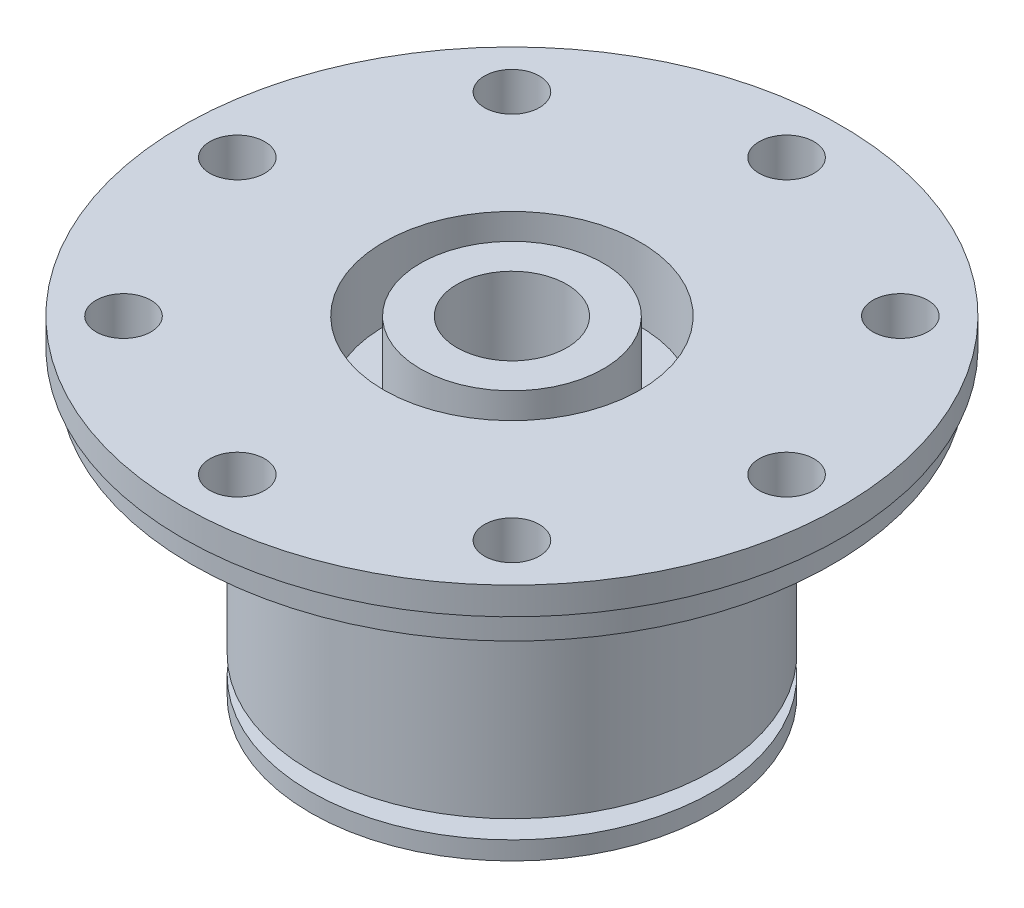
ISO-10303-21;
HEADER;
FILE_DESCRIPTION(('STEP AP214'),'2;1');
FILE_NAME('part.step','',(''),(''),'','','');
FILE_SCHEMA(('AUTOMOTIVE_DESIGN { 1 0 10303 214 1 1 1 1 }'));
ENDSEC;
DATA;
#1=APPLICATION_CONTEXT('core data for automotive mechanical design processes');
#2=APPLICATION_PROTOCOL_DEFINITION('international standard','automotive_design',2000,#1);
#3=PRODUCT_CONTEXT('',#1,'mechanical');
#4=PRODUCT('Part','Part','',(#3));
#5=PRODUCT_RELATED_PRODUCT_CATEGORY('part','',(#4));
#6=PRODUCT_DEFINITION_FORMATION('','',#4);
#7=PRODUCT_DEFINITION_CONTEXT('part definition',#1,'design');
#8=PRODUCT_DEFINITION('design','',#6,#7);
#9=PRODUCT_DEFINITION_SHAPE('','',#8);
#10=(LENGTH_UNIT() NAMED_UNIT(*) SI_UNIT(.MILLI.,.METRE.));
#11=(NAMED_UNIT(*) PLANE_ANGLE_UNIT() SI_UNIT($,.RADIAN.));
#12=(NAMED_UNIT(*) SI_UNIT($,.STERADIAN.) SOLID_ANGLE_UNIT());
#13=UNCERTAINTY_MEASURE_WITH_UNIT(LENGTH_MEASURE(1.E-05),#10,'distance_accuracy_value','');
#14=(GEOMETRIC_REPRESENTATION_CONTEXT(3) GLOBAL_UNCERTAINTY_ASSIGNED_CONTEXT((#13)) GLOBAL_UNIT_ASSIGNED_CONTEXT((#10,
#11,#12)) REPRESENTATION_CONTEXT('',''));
#15=CARTESIAN_POINT('',(0.,0.,0.));
#16=DIRECTION('',(0.,0.,1.));
#17=DIRECTION('',(1.,0.,0.));
#18=AXIS2_PLACEMENT_3D('',#15,#16,#17);
#19=CARTESIAN_POINT('',(-3.,7.42,-3.));
#20=DIRECTION('',(0.,1.,0.));
#21=DIRECTION('',(0.,0.,1.));
#22=AXIS2_PLACEMENT_3D('',#19,#20,#21);
#23=PLANE('',#22);
#24=DIRECTION('',(-1.,0.,0.));
#25=VECTOR('',#24,1.);
#26=CARTESIAN_POINT('',(-3.,7.42,3.));
#27=LINE('',#26,#25);
#28=CARTESIAN_POINT('',(3.,7.42,3.));
#29=VERTEX_POINT('',#28);
#30=CARTESIAN_POINT('',(0.,7.42,3.));
#31=VERTEX_POINT('',#30);
#32=EDGE_CURVE('E106',#29,#31,#27,.T.);
#33=ORIENTED_EDGE('',*,*,#32,.T.);
#34=CARTESIAN_POINT('',(0.,7.42,0.));
#35=DIRECTION('',(0.,1.,0.));
#36=DIRECTION('',(0.,0.,1.));
#37=AXIS2_PLACEMENT_3D('',#34,#35,#36);
#38=CIRCLE('',#37,3.);
#39=CARTESIAN_POINT('',(3.,7.42,0.));
#40=VERTEX_POINT('',#39);
#41=EDGE_CURVE('E53',#31,#40,#38,.T.);
#42=ORIENTED_EDGE('',*,*,#41,.T.);
#43=DIRECTION('',(0.,0.,1.));
#44=VECTOR('',#43,1.);
#45=CARTESIAN_POINT('',(3.,7.42,-3.));
#46=LINE('',#45,#44);
#47=EDGE_CURVE('E104',#40,#29,#46,.T.);
#48=ORIENTED_EDGE('',*,*,#47,.T.);
#49=EDGE_LOOP('',(#33,#42,#48));
#50=FACE_BOUND('',#49,.T.);
#51=ADVANCED_FACE('F39',(#50),#23,.F.);
#52=CARTESIAN_POINT('',(3.,7.42,-3.));
#53=VERTEX_POINT('',#52);
#54=EDGE_CURVE('E112',#53,#40,#46,.T.);
#55=ORIENTED_EDGE('',*,*,#54,.T.);
#56=CARTESIAN_POINT('',(0.,7.42,-3.));
#57=VERTEX_POINT('',#56);
#58=EDGE_CURVE('E95',#40,#57,#38,.T.);
#59=ORIENTED_EDGE('',*,*,#58,.T.);
#60=DIRECTION('',(-1.,0.,0.));
#61=VECTOR('',#60,1.);
#62=CARTESIAN_POINT('',(-3.,7.42,-3.));
#63=LINE('',#62,#61);
#64=EDGE_CURVE('E117',#53,#57,#63,.T.);
#65=ORIENTED_EDGE('',*,*,#64,.F.);
#66=EDGE_LOOP('',(#55,#59,#65));
#67=FACE_BOUND('',#66,.T.);
#68=ADVANCED_FACE('F111',(#67),#23,.F.);
#69=CARTESIAN_POINT('',(-3.,7.42,-3.));
#70=VERTEX_POINT('',#69);
#71=EDGE_CURVE('E208',#57,#70,#63,.T.);
#72=ORIENTED_EDGE('',*,*,#71,.F.);
#73=CARTESIAN_POINT('',(-3.,7.42,0.));
#74=VERTEX_POINT('',#73);
#75=EDGE_CURVE('E96',#57,#74,#38,.T.);
#76=ORIENTED_EDGE('',*,*,#75,.T.);
#77=DIRECTION('',(0.,0.,1.));
#78=VECTOR('',#77,1.);
#79=CARTESIAN_POINT('',(-3.,7.42,-3.));
#80=LINE('',#79,#78);
#81=EDGE_CURVE('E116',#70,#74,#80,.T.);
#82=ORIENTED_EDGE('',*,*,#81,.F.);
#83=EDGE_LOOP('',(#72,#76,#82));
#84=FACE_BOUND('',#83,.T.);
#85=ADVANCED_FACE('F184',(#84),#23,.F.);
#86=CARTESIAN_POINT('',(0.,1.,0.));
#87=DIRECTION('',(0.,-1.,0.));
#88=DIRECTION('',(0.,0.,-1.));
#89=AXIS2_PLACEMENT_3D('',#86,#87,#88);
#90=CYLINDRICAL_SURFACE('',#89,11.);
#91=CARTESIAN_POINT('',(0.,1.,0.));
#92=DIRECTION('',(0.,1.,0.));
#93=DIRECTION('',(0.,0.,1.));
#94=AXIS2_PLACEMENT_3D('',#91,#92,#93);
#95=CIRCLE('',#94,11.);
#96=CARTESIAN_POINT('',(0.,1.,11.));
#97=VERTEX_POINT('',#96);
#98=EDGE_CURVE('E152',#97,#97,#95,.T.);
#99=ORIENTED_EDGE('',*,*,#98,.F.);
#100=EDGE_LOOP('',(#99));
#101=FACE_BOUND('',#100,.T.);
#102=CARTESIAN_POINT('',(0.,0.,0.));
#103=DIRECTION('',(0.,1.,0.));
#104=DIRECTION('',(0.,0.,1.));
#105=AXIS2_PLACEMENT_3D('',#102,#103,#104);
#106=CIRCLE('',#105,11.);
#107=CARTESIAN_POINT('',(0.,0.,11.));
#108=VERTEX_POINT('',#107);
#109=EDGE_CURVE('E151',#108,#108,#106,.T.);
#110=ORIENTED_EDGE('',*,*,#109,.T.);
#111=EDGE_LOOP('',(#110));
#112=FACE_BOUND('',#111,.T.);
#113=ADVANCED_FACE('F41',(#101,#112),#90,.T.);
#114=CARTESIAN_POINT('',(0.,1.,0.));
#115=DIRECTION('',(0.,1.,0.));
#116=DIRECTION('',(0.,0.,1.));
#117=AXIS2_PLACEMENT_3D('',#114,#115,#116);
#118=PLANE('',#117);
#119=CARTESIAN_POINT('',(0.,1.,0.));
#120=DIRECTION('',(0.,1.,0.));
#121=DIRECTION('',(0.,0.,1.));
#122=AXIS2_PLACEMENT_3D('',#119,#120,#121);
#123=CIRCLE('',#122,9.5);
#124=CARTESIAN_POINT('',(0.,1.,9.5));
#125=VERTEX_POINT('',#124);
#126=EDGE_CURVE('E50',#125,#125,#123,.T.);
#127=ORIENTED_EDGE('',*,*,#126,.F.);
#128=EDGE_LOOP('',(#127));
#129=FACE_BOUND('',#128,.T.);
#130=ORIENTED_EDGE('',*,*,#98,.T.);
#131=EDGE_LOOP('',(#130));
#132=FACE_BOUND('',#131,.T.);
#133=ADVANCED_FACE('F162',(#129,#132),#118,.T.);
#134=CARTESIAN_POINT('',(0.,0.,0.));
#135=DIRECTION('',(0.,1.,0.));
#136=DIRECTION('',(0.,0.,1.));
#137=AXIS2_PLACEMENT_3D('',#134,#135,#136);
#138=PLANE('',#137);
#139=DIRECTION('',(0.,0.,1.));
#140=VECTOR('',#139,1.);
#141=CARTESIAN_POINT('',(8.,0.,-3.));
#142=LINE('',#141,#140);
#143=CARTESIAN_POINT('',(8.,0.,-3.));
#144=VERTEX_POINT('',#143);
#145=CARTESIAN_POINT('',(8.00000090304524,0.,3.));
#146=VERTEX_POINT('',#145);
#147=EDGE_CURVE('E128',#144,#146,#142,.T.);
#148=ORIENTED_EDGE('',*,*,#147,.F.);
#149=DIRECTION('',(1.,0.,0.));
#150=VECTOR('',#149,1.);
#151=CARTESIAN_POINT('',(-8.,0.,-3.));
#152=LINE('',#151,#150);
#153=CARTESIAN_POINT('',(-8.,0.,-3.));
#154=VERTEX_POINT('',#153);
#155=EDGE_CURVE('E115',#154,#144,#152,.T.);
#156=ORIENTED_EDGE('',*,*,#155,.F.);
#157=DIRECTION('',(0.,0.,1.));
#158=VECTOR('',#157,1.);
#159=CARTESIAN_POINT('',(-8.,0.,-3.));
#160=LINE('',#159,#158);
#161=CARTESIAN_POINT('',(-8.,0.,3.));
#162=VERTEX_POINT('',#161);
#163=EDGE_CURVE('E228',#154,#162,#160,.T.);
#164=ORIENTED_EDGE('',*,*,#163,.T.);
#165=DIRECTION('',(1.,0.,0.));
#166=VECTOR('',#165,1.);
#167=CARTESIAN_POINT('',(-8.,0.,3.));
#168=LINE('',#167,#166);
#169=EDGE_CURVE('E229',#162,#146,#168,.T.);
#170=ORIENTED_EDGE('',*,*,#169,.T.);
#171=EDGE_LOOP('',(#148,#156,#164,#170));
#172=FACE_BOUND('',#171,.T.);
#173=ORIENTED_EDGE('',*,*,#109,.F.);
#174=EDGE_LOOP('',(#173));
#175=FACE_BOUND('',#174,.T.);
#176=ADVANCED_FACE('F159',(#172,#175),#138,.F.);
#177=CARTESIAN_POINT('',(0.,2.,0.));
#178=DIRECTION('',(0.,-1.,0.));
#179=DIRECTION('',(0.,0.,-1.));
#180=AXIS2_PLACEMENT_3D('',#177,#178,#179);
#181=CYLINDRICAL_SURFACE('',#180,9.5);
#182=CARTESIAN_POINT('',(0.,2.,0.));
#183=DIRECTION('',(0.,1.,0.));
#184=DIRECTION('',(0.,0.,1.));
#185=AXIS2_PLACEMENT_3D('',#182,#183,#184);
#186=CIRCLE('',#185,9.5);
#187=CARTESIAN_POINT('',(0.,2.,9.5));
#188=VERTEX_POINT('',#187);
#189=EDGE_CURVE('E148',#188,#188,#186,.T.);
#190=ORIENTED_EDGE('',*,*,#189,.F.);
#191=EDGE_LOOP('',(#190));
#192=FACE_BOUND('',#191,.T.);
#193=ORIENTED_EDGE('',*,*,#126,.T.);
#194=EDGE_LOOP('',(#193));
#195=FACE_BOUND('',#194,.T.);
#196=ADVANCED_FACE('F165',(#192,#195),#181,.T.);
#197=CARTESIAN_POINT('',(0.,14.,0.));
#198=DIRECTION('',(0.,-1.,0.));
#199=DIRECTION('',(0.,0.,-1.));
#200=AXIS2_PLACEMENT_3D('',#197,#198,#199);
#201=CYLINDRICAL_SURFACE('',#200,11.);
#202=CARTESIAN_POINT('',(0.,14.,0.));
#203=DIRECTION('',(0.,1.,0.));
#204=DIRECTION('',(0.,0.,1.));
#205=AXIS2_PLACEMENT_3D('',#202,#203,#204);
#206=CIRCLE('',#205,11.);
#207=CARTESIAN_POINT('',(0.,14.,11.));
#208=VERTEX_POINT('',#207);
#209=EDGE_CURVE('E141',#208,#208,#206,.T.);
#210=ORIENTED_EDGE('',*,*,#209,.F.);
#211=EDGE_LOOP('',(#210));
#212=FACE_BOUND('',#211,.T.);
#213=CARTESIAN_POINT('',(0.,2.,0.));
#214=DIRECTION('',(0.,1.,0.));
#215=DIRECTION('',(0.,0.,1.));
#216=AXIS2_PLACEMENT_3D('',#213,#214,#215);
#217=CIRCLE('',#216,11.);
#218=CARTESIAN_POINT('',(0.,2.,11.));
#219=VERTEX_POINT('',#218);
#220=EDGE_CURVE('E136',#219,#219,#217,.T.);
#221=ORIENTED_EDGE('',*,*,#220,.T.);
#222=EDGE_LOOP('',(#221));
#223=FACE_BOUND('',#222,.T.);
#224=ADVANCED_FACE('F168',(#212,#223),#201,.T.);
#225=CARTESIAN_POINT('',(0.,2.,0.));
#226=DIRECTION('',(0.,1.,0.));
#227=DIRECTION('',(0.,0.,1.));
#228=AXIS2_PLACEMENT_3D('',#225,#226,#227);
#229=PLANE('',#228);
#230=ORIENTED_EDGE('',*,*,#189,.T.);
#231=EDGE_LOOP('',(#230));
#232=FACE_BOUND('',#231,.T.);
#233=ORIENTED_EDGE('',*,*,#220,.F.);
#234=EDGE_LOOP('',(#233));
#235=FACE_BOUND('',#234,.T.);
#236=ADVANCED_FACE('F511',(#232,#235),#229,.F.);
#237=CARTESIAN_POINT('',(0.,15.,0.));
#238=DIRECTION('',(0.,-1.,0.));
#239=DIRECTION('',(0.,0.,-1.));
#240=AXIS2_PLACEMENT_3D('',#237,#238,#239);
#241=CYLINDRICAL_SURFACE('',#240,12.);
#242=CARTESIAN_POINT('',(0.,15.,0.));
#243=DIRECTION('',(0.,1.,0.));
#244=DIRECTION('',(0.,0.,1.));
#245=AXIS2_PLACEMENT_3D('',#242,#243,#244);
#246=CIRCLE('',#245,12.);
#247=CARTESIAN_POINT('',(0.,15.,12.));
#248=VERTEX_POINT('',#247);
#249=EDGE_CURVE('E139',#248,#248,#246,.T.);
#250=ORIENTED_EDGE('',*,*,#249,.F.);
#251=EDGE_LOOP('',(#250));
#252=FACE_BOUND('',#251,.T.);
#253=CARTESIAN_POINT('',(0.,14.,0.));
#254=DIRECTION('',(0.,1.,0.));
#255=DIRECTION('',(0.,0.,1.));
#256=AXIS2_PLACEMENT_3D('',#253,#254,#255);
#257=CIRCLE('',#256,12.);
#258=CARTESIAN_POINT('',(0.,14.,12.));
#259=VERTEX_POINT('',#258);
#260=EDGE_CURVE('E131',#259,#259,#257,.T.);
#261=ORIENTED_EDGE('',*,*,#260,.T.);
#262=EDGE_LOOP('',(#261));
#263=FACE_BOUND('',#262,.T.);
#264=ADVANCED_FACE('F501',(#252,#263),#241,.T.);
#265=CARTESIAN_POINT('',(0.,14.,0.));
#266=DIRECTION('',(0.,1.,0.));
#267=DIRECTION('',(0.,0.,1.));
#268=AXIS2_PLACEMENT_3D('',#265,#266,#267);
#269=PLANE('',#268);
#270=ORIENTED_EDGE('',*,*,#209,.T.);
#271=EDGE_LOOP('',(#270));
#272=FACE_BOUND('',#271,.T.);
#273=ORIENTED_EDGE('',*,*,#260,.F.);
#274=EDGE_LOOP('',(#273));
#275=FACE_BOUND('',#274,.T.);
#276=ADVANCED_FACE('F494',(#272,#275),#269,.F.);
#277=CARTESIAN_POINT('',(0.,16.5,0.));
#278=DIRECTION('',(0.,-1.,0.));
#279=DIRECTION('',(0.,0.,-1.));
#280=AXIS2_PLACEMENT_3D('',#277,#278,#279);
#281=CYLINDRICAL_SURFACE('',#280,17.5);
#282=CARTESIAN_POINT('',(0.,16.5,0.));
#283=DIRECTION('',(0.,1.,0.));
#284=DIRECTION('',(0.,0.,1.));
#285=AXIS2_PLACEMENT_3D('',#282,#283,#284);
#286=CIRCLE('',#285,17.5);
#287=CARTESIAN_POINT('',(0.,16.5,17.5));
#288=VERTEX_POINT('',#287);
#289=EDGE_CURVE('E132',#288,#288,#286,.T.);
#290=ORIENTED_EDGE('',*,*,#289,.F.);
#291=EDGE_LOOP('',(#290));
#292=FACE_BOUND('',#291,.T.);
#293=CARTESIAN_POINT('',(0.,15.,0.));
#294=DIRECTION('',(0.,1.,0.));
#295=DIRECTION('',(0.,0.,1.));
#296=AXIS2_PLACEMENT_3D('',#293,#294,#295);
#297=CIRCLE('',#296,17.5);
#298=CARTESIAN_POINT('',(0.,15.,17.5));
#299=VERTEX_POINT('',#298);
#300=EDGE_CURVE('E127',#299,#299,#297,.T.);
#301=ORIENTED_EDGE('',*,*,#300,.T.);
#302=EDGE_LOOP('',(#301));
#303=FACE_BOUND('',#302,.T.);
#304=ADVANCED_FACE('F490',(#292,#303),#281,.T.);
#305=CARTESIAN_POINT('',(0.,15.,0.));
#306=DIRECTION('',(0.,1.,0.));
#307=DIRECTION('',(0.,0.,1.));
#308=AXIS2_PLACEMENT_3D('',#305,#306,#307);
#309=PLANE('',#308);
#310=CARTESIAN_POINT('',(0.,15.,-15.));
#311=DIRECTION('',(0.,1.,0.));
#312=DIRECTION('',(0.,0.,1.));
#313=AXIS2_PLACEMENT_3D('',#310,#311,#312);
#314=CIRCLE('',#313,1.5);
#315=CARTESIAN_POINT('',(0.,15.,-13.5));
#316=VERTEX_POINT('',#315);
#317=EDGE_CURVE('E224',#316,#316,#314,.T.);
#318=ORIENTED_EDGE('',*,*,#317,.T.);
#319=EDGE_LOOP('',(#318));
#320=FACE_BOUND('',#319,.T.);
#321=CARTESIAN_POINT('',(10.6066017177984,15.,-10.6066017177987));
#322=DIRECTION('',(0.,1.,0.));
#323=DIRECTION('',(0.,0.,1.));
#324=AXIS2_PLACEMENT_3D('',#321,#322,#323);
#325=CIRCLE('',#324,1.50000000000007);
#326=CARTESIAN_POINT('',(10.6066017177984,15.,-9.10660171779859));
#327=VERTEX_POINT('',#326);
#328=EDGE_CURVE('E286',#327,#327,#325,.T.);
#329=ORIENTED_EDGE('',*,*,#328,.T.);
#330=EDGE_LOOP('',(#329));
#331=FACE_BOUND('',#330,.T.);
#332=CARTESIAN_POINT('',(15.0000000000006,15.,-6.36733006886009E-13));
#333=DIRECTION('',(0.,1.,0.));
#334=DIRECTION('',(0.,0.,1.));
#335=AXIS2_PLACEMENT_3D('',#332,#333,#334);
#336=CIRCLE('',#335,1.50000000000047);
#337=CARTESIAN_POINT('',(15.0000000000006,15.,1.49999999999984));
#338=VERTEX_POINT('',#337);
#339=EDGE_CURVE('E289',#338,#338,#336,.T.);
#340=ORIENTED_EDGE('',*,*,#339,.T.);
#341=EDGE_LOOP('',(#340));
#342=FACE_BOUND('',#341,.T.);
#343=CARTESIAN_POINT('',(10.6066017177993,15.,10.6066017177978));
#344=DIRECTION('',(0.,1.,0.));
#345=DIRECTION('',(0.,0.,1.));
#346=AXIS2_PLACEMENT_3D('',#343,#344,#345);
#347=CIRCLE('',#346,1.50000000000098);
#348=CARTESIAN_POINT('',(10.6066017177993,15.,12.1066017177987));
#349=VERTEX_POINT('',#348);
#350=EDGE_CURVE('E281',#349,#349,#347,.T.);
#351=ORIENTED_EDGE('',*,*,#350,.T.);
#352=EDGE_LOOP('',(#351));
#353=FACE_BOUND('',#352,.T.);
#354=CARTESIAN_POINT('',(1.27346601377202E-12,15.,15.));
#355=DIRECTION('',(0.,1.,0.));
#356=DIRECTION('',(0.,0.,1.));
#357=AXIS2_PLACEMENT_3D('',#354,#355,#356);
#358=CIRCLE('',#357,1.50000000000132);
#359=CARTESIAN_POINT('',(1.27346601377202E-12,15.,16.5000000000013));
#360=VERTEX_POINT('',#359);
#361=EDGE_CURVE('E282',#360,#360,#358,.T.);
#362=ORIENTED_EDGE('',*,*,#361,.T.);
#363=EDGE_LOOP('',(#362));
#364=FACE_BOUND('',#363,.T.);
#365=CARTESIAN_POINT('',(-10.6066017177971,15.,10.6066017177987));
#366=DIRECTION('',(0.,1.,0.));
#367=DIRECTION('',(0.,0.,1.));
#368=AXIS2_PLACEMENT_3D('',#365,#366,#367);
#369=CIRCLE('',#368,1.5000000000013);
#370=CARTESIAN_POINT('',(-10.6066017177971,15.,12.1066017178));
#371=VERTEX_POINT('',#370);
#372=EDGE_CURVE('E279',#371,#371,#369,.T.);
#373=ORIENTED_EDGE('',*,*,#372,.T.);
#374=EDGE_LOOP('',(#373));
#375=FACE_BOUND('',#374,.T.);
#376=CARTESIAN_POINT('',(-14.9999999999994,15.,6.3856997708473E-13));
#377=DIRECTION('',(0.,1.,0.));
#378=DIRECTION('',(0.,0.,1.));
#379=AXIS2_PLACEMENT_3D('',#376,#377,#378);
#380=CIRCLE('',#379,1.50000000000095);
#381=CARTESIAN_POINT('',(-14.9999999999994,15.,1.50000000000159));
#382=VERTEX_POINT('',#381);
#383=EDGE_CURVE('E274',#382,#382,#380,.T.);
#384=ORIENTED_EDGE('',*,*,#383,.T.);
#385=EDGE_LOOP('',(#384));
#386=FACE_BOUND('',#385,.T.);
#387=CARTESIAN_POINT('',(-10.606601717798,15.,-10.6066017177978));
#388=DIRECTION('',(0.,1.,0.));
#389=DIRECTION('',(0.,0.,1.));
#390=AXIS2_PLACEMENT_3D('',#387,#388,#389);
#391=CIRCLE('',#390,1.50000000000049);
#392=CARTESIAN_POINT('',(-10.606601717798,15.,-9.10660171779727));
#393=VERTEX_POINT('',#392);
#394=EDGE_CURVE('E252',#393,#393,#391,.T.);
#395=ORIENTED_EDGE('',*,*,#394,.T.);
#396=EDGE_LOOP('',(#395));
#397=FACE_BOUND('',#396,.T.);
#398=ORIENTED_EDGE('',*,*,#249,.T.);
#399=EDGE_LOOP('',(#398));
#400=FACE_BOUND('',#399,.T.);
#401=ORIENTED_EDGE('',*,*,#300,.F.);
#402=EDGE_LOOP('',(#401));
#403=FACE_BOUND('',#402,.T.);
#404=ADVANCED_FACE('F293',(#320,#331,#342,#353,#364,#375,#386,#397,#400,#403),#309,.F.);
#405=CARTESIAN_POINT('',(0.,18.,0.));
#406=DIRECTION('',(0.,-1.,0.));
#407=DIRECTION('',(0.,0.,-1.));
#408=AXIS2_PLACEMENT_3D('',#405,#406,#407);
#409=CYLINDRICAL_SURFACE('',#408,18.);
#410=CARTESIAN_POINT('',(0.,18.,0.));
#411=DIRECTION('',(0.,1.,0.));
#412=DIRECTION('',(0.,0.,1.));
#413=AXIS2_PLACEMENT_3D('',#410,#411,#412);
#414=CIRCLE('',#413,18.);
#415=CARTESIAN_POINT('',(0.,18.,18.));
#416=VERTEX_POINT('',#415);
#417=EDGE_CURVE('E122',#416,#416,#414,.T.);
#418=ORIENTED_EDGE('',*,*,#417,.F.);
#419=EDGE_LOOP('',(#418));
#420=FACE_BOUND('',#419,.T.);
#421=CARTESIAN_POINT('',(0.,16.5,0.));
#422=DIRECTION('',(0.,1.,0.));
#423=DIRECTION('',(0.,0.,1.));
#424=AXIS2_PLACEMENT_3D('',#421,#422,#423);
#425=CIRCLE('',#424,18.);
#426=CARTESIAN_POINT('',(0.,16.5,18.));
#427=VERTEX_POINT('',#426);
#428=EDGE_CURVE('E130',#427,#427,#425,.T.);
#429=ORIENTED_EDGE('',*,*,#428,.T.);
#430=EDGE_LOOP('',(#429));
#431=FACE_BOUND('',#430,.T.);
#432=ADVANCED_FACE('F473',(#420,#431),#409,.T.);
#433=CARTESIAN_POINT('',(0.,18.,0.));
#434=DIRECTION('',(0.,1.,0.));
#435=DIRECTION('',(0.,0.,1.));
#436=AXIS2_PLACEMENT_3D('',#433,#434,#435);
#437=PLANE('',#436);
#438=CARTESIAN_POINT('',(0.,18.,0.));
#439=DIRECTION('',(0.,1.,0.));
#440=DIRECTION('',(0.,0.,1.));
#441=AXIS2_PLACEMENT_3D('',#438,#439,#440);
#442=CIRCLE('',#441,7.);
#443=CARTESIAN_POINT('',(0.,18.,7.));
#444=VERTEX_POINT('',#443);
#445=EDGE_CURVE('E244',#444,#444,#442,.T.);
#446=ORIENTED_EDGE('',*,*,#445,.F.);
#447=EDGE_LOOP('',(#446));
#448=FACE_BOUND('',#447,.T.);
#449=CARTESIAN_POINT('',(0.,18.,-15.));
#450=DIRECTION('',(0.,1.,0.));
#451=DIRECTION('',(0.,0.,1.));
#452=AXIS2_PLACEMENT_3D('',#449,#450,#451);
#453=CIRCLE('',#452,1.5);
#454=CARTESIAN_POINT('',(0.,18.,-13.5));
#455=VERTEX_POINT('',#454);
#456=EDGE_CURVE('E250',#455,#455,#453,.T.);
#457=ORIENTED_EDGE('',*,*,#456,.F.);
#458=EDGE_LOOP('',(#457));
#459=FACE_BOUND('',#458,.T.);
#460=CARTESIAN_POINT('',(10.6066017177984,18.,-10.6066017177987));
#461=DIRECTION('',(0.,1.,0.));
#462=DIRECTION('',(0.,0.,1.));
#463=AXIS2_PLACEMENT_3D('',#460,#461,#462);
#464=CIRCLE('',#463,1.50000000000007);
#465=CARTESIAN_POINT('',(10.6066017177984,18.,-9.10660171779859));
#466=VERTEX_POINT('',#465);
#467=EDGE_CURVE('E251',#466,#466,#464,.T.);
#468=ORIENTED_EDGE('',*,*,#467,.F.);
#469=EDGE_LOOP('',(#468));
#470=FACE_BOUND('',#469,.T.);
#471=CARTESIAN_POINT('',(15.0000000000006,18.,-6.36733006886009E-13));
#472=DIRECTION('',(0.,1.,0.));
#473=DIRECTION('',(0.,0.,1.));
#474=AXIS2_PLACEMENT_3D('',#471,#472,#473);
#475=CIRCLE('',#474,1.50000000000047);
#476=CARTESIAN_POINT('',(15.0000000000006,18.,1.49999999999984));
#477=VERTEX_POINT('',#476);
#478=EDGE_CURVE('E258',#477,#477,#475,.T.);
#479=ORIENTED_EDGE('',*,*,#478,.F.);
#480=EDGE_LOOP('',(#479));
#481=FACE_BOUND('',#480,.T.);
#482=CARTESIAN_POINT('',(10.6066017177993,18.,10.6066017177978));
#483=DIRECTION('',(0.,1.,0.));
#484=DIRECTION('',(0.,0.,1.));
#485=AXIS2_PLACEMENT_3D('',#482,#483,#484);
#486=CIRCLE('',#485,1.50000000000098);
#487=CARTESIAN_POINT('',(10.6066017177993,18.,12.1066017177987));
#488=VERTEX_POINT('',#487);
#489=EDGE_CURVE('E259',#488,#488,#486,.T.);
#490=ORIENTED_EDGE('',*,*,#489,.F.);
#491=EDGE_LOOP('',(#490));
#492=FACE_BOUND('',#491,.T.);
#493=CARTESIAN_POINT('',(1.27346601377202E-12,18.,15.));
#494=DIRECTION('',(0.,1.,0.));
#495=DIRECTION('',(0.,0.,1.));
#496=AXIS2_PLACEMENT_3D('',#493,#494,#495);
#497=CIRCLE('',#496,1.50000000000132);
#498=CARTESIAN_POINT('',(1.27346601377202E-12,18.,16.5000000000013));
#499=VERTEX_POINT('',#498);
#500=EDGE_CURVE('E265',#499,#499,#497,.T.);
#501=ORIENTED_EDGE('',*,*,#500,.F.);
#502=EDGE_LOOP('',(#501));
#503=FACE_BOUND('',#502,.T.);
#504=CARTESIAN_POINT('',(-10.6066017177971,18.,10.6066017177987));
#505=DIRECTION('',(0.,1.,0.));
#506=DIRECTION('',(0.,0.,1.));
#507=AXIS2_PLACEMENT_3D('',#504,#505,#506);
#508=CIRCLE('',#507,1.5000000000013);
#509=CARTESIAN_POINT('',(-10.6066017177971,18.,12.1066017178));
#510=VERTEX_POINT('',#509);
#511=EDGE_CURVE('E264',#510,#510,#508,.T.);
#512=ORIENTED_EDGE('',*,*,#511,.F.);
#513=EDGE_LOOP('',(#512));
#514=FACE_BOUND('',#513,.T.);
#515=CARTESIAN_POINT('',(-14.9999999999994,18.,6.3856997708473E-13));
#516=DIRECTION('',(0.,1.,0.));
#517=DIRECTION('',(0.,0.,1.));
#518=AXIS2_PLACEMENT_3D('',#515,#516,#517);
#519=CIRCLE('',#518,1.50000000000095);
#520=CARTESIAN_POINT('',(-14.9999999999994,18.,1.50000000000159));
#521=VERTEX_POINT('',#520);
#522=EDGE_CURVE('E268',#521,#521,#519,.T.);
#523=ORIENTED_EDGE('',*,*,#522,.F.);
#524=EDGE_LOOP('',(#523));
#525=FACE_BOUND('',#524,.T.);
#526=CARTESIAN_POINT('',(-10.606601717798,18.,-10.6066017177978));
#527=DIRECTION('',(0.,1.,0.));
#528=DIRECTION('',(0.,0.,1.));
#529=AXIS2_PLACEMENT_3D('',#526,#527,#528);
#530=CIRCLE('',#529,1.50000000000049);
#531=CARTESIAN_POINT('',(-10.606601717798,18.,-9.10660171779727));
#532=VERTEX_POINT('',#531);
#533=EDGE_CURVE('E248',#532,#532,#530,.T.);
#534=ORIENTED_EDGE('',*,*,#533,.F.);
#535=EDGE_LOOP('',(#534));
#536=FACE_BOUND('',#535,.T.);
#537=ORIENTED_EDGE('',*,*,#417,.T.);
#538=EDGE_LOOP('',(#537));
#539=FACE_BOUND('',#538,.T.);
#540=ADVANCED_FACE('F465',(#448,#459,#470,#481,#492,#503,#514,#525,#536,#539),#437,.T.);
#541=CARTESIAN_POINT('',(0.,16.5,0.));
#542=DIRECTION('',(0.,1.,0.));
#543=DIRECTION('',(0.,0.,1.));
#544=AXIS2_PLACEMENT_3D('',#541,#542,#543);
#545=PLANE('',#544);
#546=ORIENTED_EDGE('',*,*,#289,.T.);
#547=EDGE_LOOP('',(#546));
#548=FACE_BOUND('',#547,.T.);
#549=ORIENTED_EDGE('',*,*,#428,.F.);
#550=EDGE_LOOP('',(#549));
#551=FACE_BOUND('',#550,.T.);
#552=ADVANCED_FACE('F460',(#548,#551),#545,.F.);
#553=CARTESIAN_POINT('',(9.03045244485257E-07,0.00380114760461332,-3.));
#554=DIRECTION('',(0.,0.,1.));
#555=DIRECTION('',(1.,0.,0.));
#556=AXIS2_PLACEMENT_3D('',#553,#554,#555);
#557=CYLINDRICAL_SURFACE('',#556,8.);
#558=CARTESIAN_POINT('',(9.03045244485257E-07,0.00380114760461332,3.));
#559=DIRECTION('',(0.,0.,1.));
#560=DIRECTION('',(-1.,0.,0.));
#561=AXIS2_PLACEMENT_3D('',#558,#559,#560);
#562=CIRCLE('',#561,8.);
#563=EDGE_CURVE('E64',#146,#29,#562,.T.);
#564=ORIENTED_EDGE('',*,*,#563,.T.);
#565=ORIENTED_EDGE('',*,*,#47,.F.);
#566=ORIENTED_EDGE('',*,*,#54,.F.);
#567=CARTESIAN_POINT('',(9.03045244485257E-07,0.00380114760461332,-3.));
#568=DIRECTION('',(0.,0.,1.));
#569=DIRECTION('',(-1.,0.,0.));
#570=AXIS2_PLACEMENT_3D('',#567,#568,#569);
#571=CIRCLE('',#570,8.);
#572=EDGE_CURVE('E215',#144,#53,#571,.T.);
#573=ORIENTED_EDGE('',*,*,#572,.F.);
#574=ORIENTED_EDGE('',*,*,#147,.T.);
#575=EDGE_LOOP('',(#564,#565,#566,#573,#574));
#576=FACE_BOUND('',#575,.T.);
#577=ADVANCED_FACE('F109',(#576),#557,.F.);
#578=CARTESIAN_POINT('',(-9.03045245352618E-07,0.00380114760461462,-3.));
#579=DIRECTION('',(0.,0.,1.));
#580=DIRECTION('',(1.,0.,0.));
#581=AXIS2_PLACEMENT_3D('',#578,#579,#580);
#582=CYLINDRICAL_SURFACE('',#581,8.);
#583=CARTESIAN_POINT('',(-9.03045245352618E-07,0.00380114760461462,3.));
#584=DIRECTION('',(0.,0.,1.));
#585=DIRECTION('',(-1.,0.,0.));
#586=AXIS2_PLACEMENT_3D('',#583,#584,#585);
#587=CIRCLE('',#586,8.);
#588=CARTESIAN_POINT('',(-3.,7.42,3.));
#589=VERTEX_POINT('',#588);
#590=EDGE_CURVE('E223',#589,#162,#587,.T.);
#591=ORIENTED_EDGE('',*,*,#590,.T.);
#592=ORIENTED_EDGE('',*,*,#163,.F.);
#593=CARTESIAN_POINT('',(-9.03045245352618E-07,0.00380114760461462,-3.));
#594=DIRECTION('',(0.,0.,1.));
#595=DIRECTION('',(-1.,0.,0.));
#596=AXIS2_PLACEMENT_3D('',#593,#594,#595);
#597=CIRCLE('',#596,8.);
#598=EDGE_CURVE('E214',#70,#154,#597,.T.);
#599=ORIENTED_EDGE('',*,*,#598,.F.);
#600=ORIENTED_EDGE('',*,*,#81,.T.);
#601=EDGE_CURVE('E120',#74,#589,#80,.T.);
#602=ORIENTED_EDGE('',*,*,#601,.T.);
#603=EDGE_LOOP('',(#591,#592,#599,#600,#602));
#604=FACE_BOUND('',#603,.T.);
#605=ADVANCED_FACE('F186',(#604),#582,.F.);
#606=ORIENTED_EDGE('',*,*,#601,.F.);
#607=EDGE_CURVE('E107',#74,#31,#38,.T.);
#608=ORIENTED_EDGE('',*,*,#607,.T.);
#609=EDGE_CURVE('E225',#31,#589,#27,.T.);
#610=ORIENTED_EDGE('',*,*,#609,.T.);
#611=EDGE_LOOP('',(#606,#608,#610));
#612=FACE_BOUND('',#611,.T.);
#613=ADVANCED_FACE('F180',(#612),#23,.F.);
#614=CARTESIAN_POINT('',(9.03045244485257E-07,0.00380114760461332,-3.));
#615=DIRECTION('',(0.,0.,-1.));
#616=DIRECTION('',(-1.,0.,0.));
#617=AXIS2_PLACEMENT_3D('',#614,#615,#616);
#618=PLANE('',#617);
#619=ORIENTED_EDGE('',*,*,#572,.T.);
#620=ORIENTED_EDGE('',*,*,#64,.T.);
#621=ORIENTED_EDGE('',*,*,#71,.T.);
#622=ORIENTED_EDGE('',*,*,#598,.T.);
#623=ORIENTED_EDGE('',*,*,#155,.T.);
#624=EDGE_LOOP('',(#619,#620,#621,#622,#623));
#625=FACE_BOUND('',#624,.T.);
#626=ADVANCED_FACE('F190',(#625),#618,.F.);
#627=CARTESIAN_POINT('',(9.03045244485257E-07,0.00380114760461332,3.));
#628=DIRECTION('',(0.,0.,-1.));
#629=DIRECTION('',(-1.,0.,0.));
#630=AXIS2_PLACEMENT_3D('',#627,#628,#629);
#631=PLANE('',#630);
#632=ORIENTED_EDGE('',*,*,#563,.F.);
#633=ORIENTED_EDGE('',*,*,#169,.F.);
#634=ORIENTED_EDGE('',*,*,#590,.F.);
#635=ORIENTED_EDGE('',*,*,#609,.F.);
#636=ORIENTED_EDGE('',*,*,#32,.F.);
#637=EDGE_LOOP('',(#632,#633,#634,#635,#636));
#638=FACE_BOUND('',#637,.T.);
#639=ADVANCED_FACE('F191',(#638),#631,.T.);
#640=CARTESIAN_POINT('',(-10.606601717798,12.,-10.6066017177978));
#641=DIRECTION('',(0.,1.,0.));
#642=DIRECTION('',(0.,0.,1.));
#643=AXIS2_PLACEMENT_3D('',#640,#641,#642);
#644=CYLINDRICAL_SURFACE('',#643,1.50000000000049);
#645=ORIENTED_EDGE('',*,*,#533,.T.);
#646=EDGE_LOOP('',(#645));
#647=FACE_BOUND('',#646,.T.);
#648=ORIENTED_EDGE('',*,*,#394,.F.);
#649=EDGE_LOOP('',(#648));
#650=FACE_BOUND('',#649,.T.);
#651=ADVANCED_FACE('F333',(#647,#650),#644,.F.);
#652=CARTESIAN_POINT('',(-14.9999999999994,12.,6.3856997708473E-13));
#653=DIRECTION('',(0.,1.,0.));
#654=DIRECTION('',(0.,0.,1.));
#655=AXIS2_PLACEMENT_3D('',#652,#653,#654);
#656=CYLINDRICAL_SURFACE('',#655,1.50000000000095);
#657=ORIENTED_EDGE('',*,*,#522,.T.);
#658=EDGE_LOOP('',(#657));
#659=FACE_BOUND('',#658,.T.);
#660=ORIENTED_EDGE('',*,*,#383,.F.);
#661=EDGE_LOOP('',(#660));
#662=FACE_BOUND('',#661,.T.);
#663=ADVANCED_FACE('F332',(#659,#662),#656,.F.);
#664=CARTESIAN_POINT('',(-10.6066017177971,12.,10.6066017177987));
#665=DIRECTION('',(0.,1.,0.));
#666=DIRECTION('',(0.,0.,1.));
#667=AXIS2_PLACEMENT_3D('',#664,#665,#666);
#668=CYLINDRICAL_SURFACE('',#667,1.5000000000013);
#669=ORIENTED_EDGE('',*,*,#511,.T.);
#670=EDGE_LOOP('',(#669));
#671=FACE_BOUND('',#670,.T.);
#672=ORIENTED_EDGE('',*,*,#372,.F.);
#673=EDGE_LOOP('',(#672));
#674=FACE_BOUND('',#673,.T.);
#675=ADVANCED_FACE('F330',(#671,#674),#668,.F.);
#676=CARTESIAN_POINT('',(1.27346601377202E-12,12.,15.));
#677=DIRECTION('',(0.,1.,0.));
#678=DIRECTION('',(0.,0.,1.));
#679=AXIS2_PLACEMENT_3D('',#676,#677,#678);
#680=CYLINDRICAL_SURFACE('',#679,1.50000000000132);
#681=ORIENTED_EDGE('',*,*,#500,.T.);
#682=EDGE_LOOP('',(#681));
#683=FACE_BOUND('',#682,.T.);
#684=ORIENTED_EDGE('',*,*,#361,.F.);
#685=EDGE_LOOP('',(#684));
#686=FACE_BOUND('',#685,.T.);
#687=ADVANCED_FACE('F323',(#683,#686),#680,.F.);
#688=CARTESIAN_POINT('',(10.6066017177993,12.,10.6066017177978));
#689=DIRECTION('',(0.,1.,0.));
#690=DIRECTION('',(0.,0.,1.));
#691=AXIS2_PLACEMENT_3D('',#688,#689,#690);
#692=CYLINDRICAL_SURFACE('',#691,1.50000000000098);
#693=ORIENTED_EDGE('',*,*,#489,.T.);
#694=EDGE_LOOP('',(#693));
#695=FACE_BOUND('',#694,.T.);
#696=ORIENTED_EDGE('',*,*,#350,.F.);
#697=EDGE_LOOP('',(#696));
#698=FACE_BOUND('',#697,.T.);
#699=ADVANCED_FACE('F317',(#695,#698),#692,.F.);
#700=CARTESIAN_POINT('',(15.0000000000006,12.,-6.36733006886009E-13));
#701=DIRECTION('',(0.,1.,0.));
#702=DIRECTION('',(0.,0.,1.));
#703=AXIS2_PLACEMENT_3D('',#700,#701,#702);
#704=CYLINDRICAL_SURFACE('',#703,1.50000000000047);
#705=ORIENTED_EDGE('',*,*,#478,.T.);
#706=EDGE_LOOP('',(#705));
#707=FACE_BOUND('',#706,.T.);
#708=ORIENTED_EDGE('',*,*,#339,.F.);
#709=EDGE_LOOP('',(#708));
#710=FACE_BOUND('',#709,.T.);
#711=ADVANCED_FACE('F315',(#707,#710),#704,.F.);
#712=CARTESIAN_POINT('',(10.6066017177984,12.,-10.6066017177987));
#713=DIRECTION('',(0.,1.,0.));
#714=DIRECTION('',(0.,0.,1.));
#715=AXIS2_PLACEMENT_3D('',#712,#713,#714);
#716=CYLINDRICAL_SURFACE('',#715,1.50000000000007);
#717=ORIENTED_EDGE('',*,*,#467,.T.);
#718=EDGE_LOOP('',(#717));
#719=FACE_BOUND('',#718,.T.);
#720=ORIENTED_EDGE('',*,*,#328,.F.);
#721=EDGE_LOOP('',(#720));
#722=FACE_BOUND('',#721,.T.);
#723=ADVANCED_FACE('F303',(#719,#722),#716,.F.);
#724=CARTESIAN_POINT('',(0.,12.,-15.));
#725=DIRECTION('',(0.,1.,0.));
#726=DIRECTION('',(0.,0.,1.));
#727=AXIS2_PLACEMENT_3D('',#724,#725,#726);
#728=CYLINDRICAL_SURFACE('',#727,1.5);
#729=ORIENTED_EDGE('',*,*,#456,.T.);
#730=EDGE_LOOP('',(#729));
#731=FACE_BOUND('',#730,.T.);
#732=ORIENTED_EDGE('',*,*,#317,.F.);
#733=EDGE_LOOP('',(#732));
#734=FACE_BOUND('',#733,.T.);
#735=ADVANCED_FACE('F300',(#731,#734),#728,.F.);
#736=CARTESIAN_POINT('',(0.,14.,0.));
#737=DIRECTION('',(0.,1.,0.));
#738=DIRECTION('',(0.,0.,1.));
#739=AXIS2_PLACEMENT_3D('',#736,#737,#738);
#740=CYLINDRICAL_SURFACE('',#739,7.);
#741=CARTESIAN_POINT('',(0.,14.,0.));
#742=DIRECTION('',(0.,1.,0.));
#743=DIRECTION('',(0.,0.,1.));
#744=AXIS2_PLACEMENT_3D('',#741,#742,#743);
#745=CIRCLE('',#744,7.);
#746=CARTESIAN_POINT('',(0.,14.,7.));
#747=VERTEX_POINT('',#746);
#748=EDGE_CURVE('E245',#747,#747,#745,.T.);
#749=ORIENTED_EDGE('',*,*,#748,.F.);
#750=EDGE_LOOP('',(#749));
#751=FACE_BOUND('',#750,.T.);
#752=ORIENTED_EDGE('',*,*,#445,.T.);
#753=EDGE_LOOP('',(#752));
#754=FACE_BOUND('',#753,.T.);
#755=ADVANCED_FACE('F298',(#751,#754),#740,.F.);
#756=CARTESIAN_POINT('',(0.,14.,0.));
#757=DIRECTION('',(0.,1.,0.));
#758=DIRECTION('',(0.,0.,1.));
#759=AXIS2_PLACEMENT_3D('',#756,#757,#758);
#760=PLANE('',#759);
#761=CARTESIAN_POINT('',(0.,14.,0.));
#762=DIRECTION('',(0.,1.,0.));
#763=DIRECTION('',(0.,0.,1.));
#764=AXIS2_PLACEMENT_3D('',#761,#762,#763);
#765=CIRCLE('',#764,5.);
#766=CARTESIAN_POINT('',(0.,14.,5.));
#767=VERTEX_POINT('',#766);
#768=EDGE_CURVE('E11',#767,#767,#765,.T.);
#769=ORIENTED_EDGE('',*,*,#768,.F.);
#770=EDGE_LOOP('',(#769));
#771=FACE_BOUND('',#770,.T.);
#772=ORIENTED_EDGE('',*,*,#748,.T.);
#773=EDGE_LOOP('',(#772));
#774=FACE_BOUND('',#773,.T.);
#775=ADVANCED_FACE('F310',(#771,#774),#760,.T.);
#776=CARTESIAN_POINT('',(0.,14.,0.));
#777=DIRECTION('',(0.,1.,0.));
#778=DIRECTION('',(0.,0.,1.));
#779=AXIS2_PLACEMENT_3D('',#776,#777,#778);
#780=CYLINDRICAL_SURFACE('',#779,5.);
#781=ORIENTED_EDGE('',*,*,#768,.T.);
#782=EDGE_LOOP('',(#781));
#783=FACE_BOUND('',#782,.T.);
#784=CARTESIAN_POINT('',(0.,18.,0.));
#785=DIRECTION('',(0.,1.,0.));
#786=DIRECTION('',(0.,0.,1.));
#787=AXIS2_PLACEMENT_3D('',#784,#785,#786);
#788=CIRCLE('',#787,5.);
#789=CARTESIAN_POINT('',(0.,18.,5.));
#790=VERTEX_POINT('',#789);
#791=EDGE_CURVE('E110',#790,#790,#788,.T.);
#792=ORIENTED_EDGE('',*,*,#791,.F.);
#793=EDGE_LOOP('',(#792));
#794=FACE_BOUND('',#793,.T.);
#795=ADVANCED_FACE('F351',(#783,#794),#780,.T.);
#796=CARTESIAN_POINT('',(0.,18.,0.));
#797=DIRECTION('',(0.,1.,0.));
#798=DIRECTION('',(0.,0.,1.));
#799=AXIS2_PLACEMENT_3D('',#796,#797,#798);
#800=PLANE('',#799);
#801=CARTESIAN_POINT('',(0.,18.,0.));
#802=DIRECTION('',(0.,1.,0.));
#803=DIRECTION('',(0.,0.,1.));
#804=AXIS2_PLACEMENT_3D('',#801,#802,#803);
#805=CIRCLE('',#804,3.);
#806=CARTESIAN_POINT('',(0.,18.,3.));
#807=VERTEX_POINT('',#806);
#808=EDGE_CURVE('E237',#807,#807,#805,.T.);
#809=ORIENTED_EDGE('',*,*,#808,.F.);
#810=EDGE_LOOP('',(#809));
#811=FACE_BOUND('',#810,.T.);
#812=ORIENTED_EDGE('',*,*,#791,.T.);
#813=EDGE_LOOP('',(#812));
#814=FACE_BOUND('',#813,.T.);
#815=ADVANCED_FACE('F348',(#811,#814),#800,.T.);
#816=CARTESIAN_POINT('',(0.,7.42,0.));
#817=DIRECTION('',(0.,1.,0.));
#818=DIRECTION('',(0.,0.,1.));
#819=AXIS2_PLACEMENT_3D('',#816,#817,#818);
#820=CYLINDRICAL_SURFACE('',#819,3.);
#821=ORIENTED_EDGE('',*,*,#41,.F.);
#822=ORIENTED_EDGE('',*,*,#607,.F.);
#823=ORIENTED_EDGE('',*,*,#75,.F.);
#824=ORIENTED_EDGE('',*,*,#58,.F.);
#825=EDGE_LOOP('',(#821,#822,#823,#824));
#826=FACE_BOUND('',#825,.T.);
#827=ORIENTED_EDGE('',*,*,#808,.T.);
#828=EDGE_LOOP('',(#827));
#829=FACE_BOUND('',#828,.T.);
#830=ADVANCED_FACE('F91',(#826,#829),#820,.F.);
#831=CLOSED_SHELL('',(#51,#68,#85,#113,#133,#176,#196,#224,#236,#264,#276,#304,#404,#432,#540,
#552,#577,#605,#613,#626,#639,#651,#663,#675,#687,#699,#711,#723,#735,#755,#775,#795,#815,#830));
#832=MANIFOLD_SOLID_BREP('B2',#831);
#833=ADVANCED_BREP_SHAPE_REPRESENTATION('',(#18,#832),#14);
#834=SHAPE_DEFINITION_REPRESENTATION(#9,#833);
ENDSEC;
END-ISO-10303-21;
